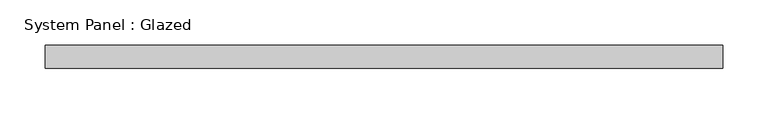
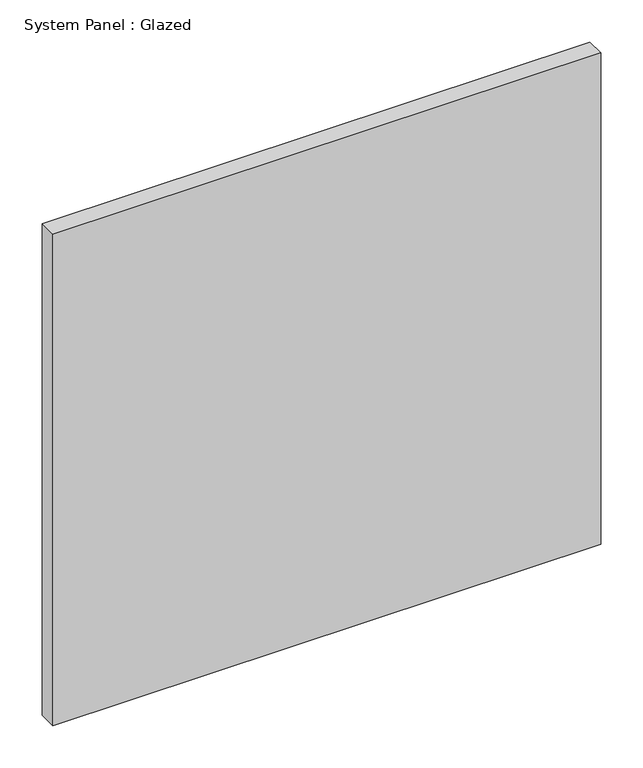
"""IFC4 building model written with IfcOpenShell, lengths in millimetres: plate geometry, System Panel : Glazed."""

from ifc_helpers import new_model, si_unit, origin, origin_with_axes, place, context, project, spatial, polyline, outline, extrude, source, transform, mapped, element, save


def system_panel_glazed_edf5bdbe(model_context):
    return source(origin(), model_context, "Body", "SweptSolid", [
        extrude(outline(polyline([(374.65, 19.05), (-374.65, 19.05), (-374.65, 44.45), (374.65, 44.45), (374.65, 19.05)])), origin_with_axes(), (0.0, 0.0, 1.0), 710.9382113),
    ])


if __name__ == "__main__":
    model = new_model("IFC4")
    model_context = context("Model", 3, world=origin())
    ifc_project = project(units=[si_unit("LENGTHUNIT", "METRE", prefix="MILLI")], contexts=[model_context])
    site = spatial("IfcSite", under=ifc_project)
    building = spatial("IfcBuilding", under=site)
    placement = place(None, origin())
    system_panel_glazed_shape = system_panel_glazed_edf5bdbe(model_context)
    element("IfcPlate", 1, ObjectType="System Panel : Glazed", at=placement, inside=building, context=model_context, shape_type="MappedRepresentation", body=[
        mapped(system_panel_glazed_shape, transform((0.0, 0.0, 0.0), x_axis=(1.0, 0.0, 0.0), y_axis=(0.0, 1.0, 0.0), z_axis=(0.0, 0.0, 1.0))),
    ])
    save(model, "model.ifc")

# Revit data of these elements
# Type "System Panel : Glazed"
#   Construction Type Id = "GSP4R"
#   Analytic Construction = "1/8 in Pilkington single glazing"
#   Visual Light Transmittance = 0.9
#   Solar Heat Gain Coefficient = 0.86
#   Heat Transfer Coefficient (U) = 1.18115 BTU/(h·ft²·°F)
#   Define Thermal Properties by = 1
# Element 1 (IfcPlate, "System Panel : Glazed")
#   Materials on its faces: "Glass"
# Materials
#   "Glass": class "Glass", colour RGB 0 128 192, transparency 0.75, Description = "Soda Lime Glass", Cost = 0
